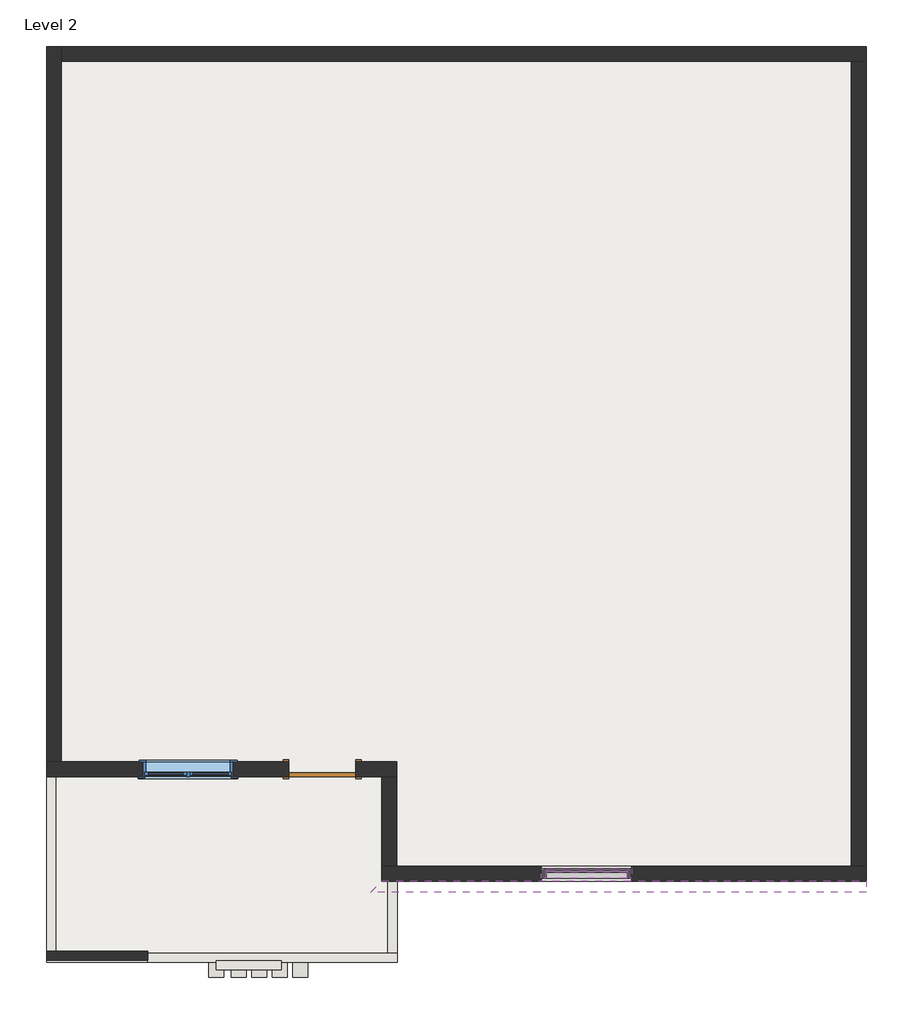
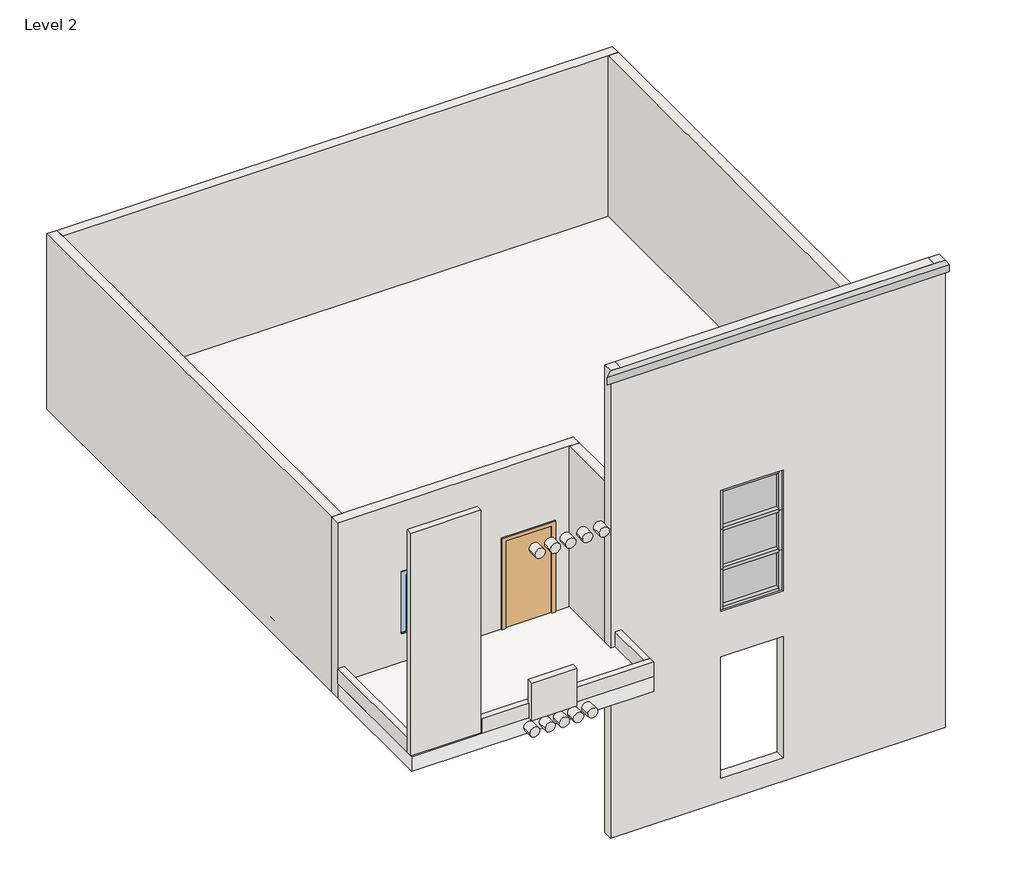
# One storey: 12 walls, 10 members, 3 plates, 1 door, 1 proxy, 1 roof, 1 window.
"""IFC4 building model written with IfcOpenShell, lengths in millimetres."""

from ifc_helpers import new_model, si_unit, frame, origin, place, context, project, spatial, polyline, outline, extrude, faceted_brep, transform, mapped, element, save
from components import door_54dd4da4, member_b365ec95, member_88401a07, member_a8c92c1b, system_panel_glazed_b873dfd1, system_panel_glazed_e970100d, walls_4_walls_4_cfa72774, window_0862ab64

model = new_model("IFC4")

# Units and contexts
model_context = context("Model", 3, world=origin())
ifc_project = project(units=[si_unit("LENGTHUNIT", "METRE", prefix="MILLI")], contexts=[model_context])

# Site, building, storey
site = spatial("IfcSite", under=ifc_project)
building = spatial("IfcBuilding", under=site)
storey = spatial("IfcBuildingStorey", under=building, Name="Level 2", Elevation=3657.6)

# Proxy
placement = place(None, origin())
element("IfcBuildingElementProxy", 1, Name="Cornice", ObjectType="Cornice", at=placement, inside=storey, context=model_context, shape_type="SweptSolid", body=[
    extrude(outline(polyline([(-6596.5183714, -375.7099629), (-6444.1183714, -223.3099629), (159.8816286, -223.3099629), (159.8816286, -375.7099629), (-6596.5183714, -375.7099629)])), frame((0.0, 0.0, 9601.2), z_axis=(0.0, 0.0, 1.0), x_axis=(1.0, 0.0, 0.0)), (0.0, 0.0, 1.0), 152.4),
])

# Door
door_shape = door_54dd4da4(model_context)
element("IfcDoor", 2, ObjectType="Single-Flush : 36\" x 84\"", at=placement, inside=storey, context=model_context, shape_type="MappedRepresentation", body=[
    mapped(door_shape, transform((-7256.9183714, 1300.6900371, 3657.6), x_axis=(-1.0, 0.0, 0.0), y_axis=(0.0, -1.0, 0.0), z_axis=(0.0, 0.0, 1.0))),
])

# Members
member_shape = member_b365ec95(model_context)
element("IfcMember", 3, ObjectType="Rectangular Mullion : 2.5\" x 5\" rectangular", at=placement, inside=storey, context=model_context, shape_type="MappedRepresentation", body=[
    mapped(member_shape, transform((-4267.1276154, -121.7099629, 5644.4580483), x_axis=(-1.0, 0.0, 0.0), y_axis=(0.0, -1.0, 0.0), z_axis=(0.0, 0.0, 1.0))),
])
element("IfcMember", 4, ObjectType="Rectangular Mullion : 2.5\" x 5\" rectangular", at=placement, inside=storey, context=model_context, shape_type="MappedRepresentation", body=[
    mapped(member_shape, transform((-4267.1276154, -121.7099629, 6485.4870724), x_axis=(-1.0, 0.0, 0.0), y_axis=(0.0, -1.0, 0.0), z_axis=(0.0, 0.0, 1.0))),
])
member_2_shape = member_88401a07(model_context)
element("IfcMember", 5, ObjectType="Rectangular Mullion : 2.5\" x 5\" rectangular", at=placement, inside=storey, context=model_context, shape_type="MappedRepresentation", body=[
    mapped(member_2_shape, transform((-3100.8433714, -121.7099629, 5644.4580483), x_axis=(0.0, 0.0, 1.0), y_axis=(0.0, -1.0, 0.0), z_axis=(1.0, 0.0, 0.0))),
])
element("IfcMember", 6, ObjectType="Rectangular Mullion : 2.5\" x 5\" rectangular", at=placement, inside=storey, context=model_context, shape_type="MappedRepresentation", body=[
    mapped(member_2_shape, transform((-3100.8433714, -121.7099629, 4803.4290241), x_axis=(0.0, 0.0, 1.0), y_axis=(0.0, -1.0, 0.0), z_axis=(1.0, 0.0, 0.0))),
])
member_3_shape = member_a8c92c1b(model_context)
element("IfcMember", 7, ObjectType="Rectangular Mullion : 2.5\" x 5\" rectangular", at=placement, inside=storey, context=model_context, shape_type="MappedRepresentation", body=[
    mapped(member_3_shape, transform((-3100.8433714, -121.7099629, 6485.4870724), x_axis=(0.0, 0.0, 1.0), y_axis=(0.0, -1.0, 0.0), z_axis=(1.0, 0.0, 0.0))),
])
element("IfcMember", 8, ObjectType="Rectangular Mullion : 2.5\" x 5\" rectangular", at=placement, inside=storey, context=model_context, shape_type="MappedRepresentation", body=[
    mapped(member_shape, transform((-3037.3433714, -121.7099629, 4803.4290241), x_axis=(1.0, 0.0, 0.0), y_axis=(0.0, -1.0, 0.0), z_axis=(0.0, 0.0, -1.0))),
])
element("IfcMember", 9, ObjectType="Rectangular Mullion : 2.5\" x 5\" rectangular", at=placement, inside=storey, context=model_context, shape_type="MappedRepresentation", body=[
    mapped(member_shape, transform((-3037.3433714, -121.7099629, 5644.4580483), x_axis=(1.0, 0.0, 0.0), y_axis=(0.0, -1.0, 0.0), z_axis=(0.0, 0.0, -1.0))),
])
element("IfcMember", 10, ObjectType="Rectangular Mullion : 2.5\" x 5\" rectangular", at=placement, inside=storey, context=model_context, shape_type="MappedRepresentation", body=[
    mapped(member_3_shape, transform((-4203.6276154, -121.7099629, 3962.4), x_axis=(0.0, 0.0, -1.0), y_axis=(0.0, -1.0, 0.0), z_axis=(-1.0, 0.0, 0.0))),
])
element("IfcMember", 11, ObjectType="Rectangular Mullion : 2.5\" x 5\" rectangular", at=placement, inside=storey, context=model_context, shape_type="MappedRepresentation", body=[
    mapped(member_shape, transform((-4267.1276154, -121.7099629, 4803.4290241), x_axis=(-1.0, 0.0, 0.0), y_axis=(0.0, -1.0, 0.0), z_axis=(0.0, 0.0, 1.0))),
])
element("IfcMember", 12, ObjectType="Rectangular Mullion : 2.5\" x 5\" rectangular", at=placement, inside=storey, context=model_context, shape_type="MappedRepresentation", body=[
    mapped(member_shape, transform((-3037.3433714, -121.7099629, 3962.4), x_axis=(1.0, 0.0, 0.0), y_axis=(0.0, -1.0, 0.0), z_axis=(0.0, 0.0, -1.0))),
])

# Plates
system_panel_glazed_shape = system_panel_glazed_b873dfd1(model_context)
element("IfcPlate", 13, ObjectType="System Panel : Glazed", at=placement, inside=storey, context=model_context, shape_type="MappedRepresentation", body=[
    mapped(system_panel_glazed_shape, transform((-3652.2354934, -121.7099629, 4025.9), x_axis=(1.0, 0.0, 0.0), y_axis=(0.0, 1.0, 0.0), z_axis=(0.0, 0.0, 1.0))),
])
element("IfcPlate", 14, ObjectType="System Panel : Glazed", at=placement, inside=storey, context=model_context, shape_type="MappedRepresentation", body=[
    mapped(system_panel_glazed_shape, transform((-3652.2354934, -121.7099629, 5676.2080483), x_axis=(1.0, 0.0, 0.0), y_axis=(0.0, 1.0, 0.0), z_axis=(0.0, 0.0, 1.0))),
])
system_panel_glazed_2_shape = system_panel_glazed_e970100d(model_context)
element("IfcPlate", 15, ObjectType="System Panel : Glazed", at=placement, inside=storey, context=model_context, shape_type="MappedRepresentation", body=[
    mapped(system_panel_glazed_2_shape, transform((-3652.2354934, -121.7099629, 4835.1790241), x_axis=(1.0, 0.0, 0.0), y_axis=(0.0, 1.0, 0.0), z_axis=(0.0, 0.0, 1.0))),
])

# Roof
element("IfcRoof", 16, ObjectType="Generic - 12\"", at=placement, inside=storey, context=model_context, shape_type="SweptSolid", body=[
    extrude(outline(polyline([(-11016.1183714, 11155.8900371), (159.8816286, 11155.8900371), (159.8816286, -20.1099629), (-6234.5683714, -20.1099629), (-6234.5683714, -1332.6895946), (-11016.1183714, -1332.6895946), (-11016.1183714, 11155.8900371)])), frame((0.0, 0.0, 3657.6), z_axis=(0.0, 0.0, 1.0), x_axis=(1.0, 0.0, 0.0)), (0.0, 0.0, 1.0), 304.8),
])

# Walls
element("IfcWall", 17, ObjectType="Generic - 5\"", at=placement, inside=storey, context=model_context, shape_type="Brep", body=[
    faceted_brep([(-11016.1183714, -1306.3008757, 8615.143067), (-11016.1183714, -1306.3008757, 3962.4), (-9633.3839949, -1306.3008757, 3962.4), (-9633.3839949, -1306.3008757, 8615.143067), (-11016.1183714, -1179.3008757, 3962.4), (-11016.1183714, -1179.3008757, 4267.2), (-11016.1183714, -1179.3008757, 7620.0), (-11016.1183714, -1179.3008757, 7924.8), (-11016.1183714, -1179.3008757, 8615.143067), (-9633.3839949, -1179.3008757, 8615.143067), (-9633.3839949, -1179.3008757, 3962.4), (-10889.1183714, -1179.3008757, 3962.4), (-9633.3839949, -1205.6895946, 3962.4)], [[[0, 1, 2, 3]], [[4, 5, 6, 7, 8, 9, 10, 11]], [[2, 1, 4, 11, 10, 12]], [[0, 3, 9, 8]], [[2, 12, 10, 9, 3]], [[0, 8, 7, 6, 5, 4, 1]]]),
])
element("IfcWall", 18, ObjectType="Generic - 5\"", at=placement, inside=storey, context=model_context, shape_type="Brep", body=[
    faceted_brep([(-9633.3839949, -1332.6895946, 3962.4), (-6234.5683714, -1332.6895946, 3962.4), (-6234.5683714, -1332.6895946, 4267.2), (-9633.3839949, -1332.6895946, 4267.2), (-9633.3839949, -1205.6895946, 3962.4), (-9633.3839949, -1205.6895946, 4267.2), (-6361.5683714, -1205.6895946, 4267.2), (-6234.5683714, -1205.6895946, 4267.2), (-6234.5683714, -1205.6895946, 3962.4), (-6361.5683714, -1205.6895946, 3962.4), (-9633.3839949, -1306.3008757, 3962.4)], [[[0, 1, 2, 3]], [[4, 5, 6, 7, 8, 9]], [[1, 0, 10, 4, 9, 8]], [[3, 2, 7, 6, 5]], [[0, 3, 5, 4, 10]], [[2, 1, 8, 7]]]),
])
element("IfcWall", 19, ObjectType="Generic - 5\"", at=placement, inside=storey, context=model_context, shape_type="SweptSolid", body=[
    extrude(outline(polyline([(-6234.5683714, -223.3099629), (-6234.5683714, -1205.6895946), (-6361.5683714, -1205.6895946), (-6361.5683714, -223.3099629), (-6234.5683714, -223.3099629)])), frame((0.0, 0.0, 3962.4), z_axis=(0.0, 0.0, 1.0), x_axis=(1.0, 0.0, 0.0)), (0.0, 0.0, 1.0), 304.8),
])
element("IfcWall", 20, ObjectType="Generic - 5\"", at=placement, inside=storey, context=model_context, shape_type="SweptSolid", body=[
    extrude(outline(polyline([(-11016.1183714, -1179.3008757), (-11016.1183714, 1199.0900371), (-10889.1183714, 1199.0900371), (-10889.1183714, -1179.3008757), (-11016.1183714, -1179.3008757)])), frame((0.0, 0.0, 3962.4), z_axis=(0.0, 0.0, 1.0), x_axis=(1.0, 0.0, 0.0)), (0.0, 0.0, 1.0), 304.8),
])
element("IfcWall", 21, ObjectType="Generic - 5\"", at=placement, inside=storey, context=model_context, shape_type="SweptSolid", body=[
    extrude(outline(polyline([(-7812.5433714, -1434.2895946), (-8701.5433714, -1434.2895946), (-8701.5433714, -1307.2895946), (-7812.5433714, -1307.2895946), (-7812.5433714, -1434.2895946)])), frame((0.0, 0.0, 3962.4), z_axis=(0.0, 0.0, 1.0), x_axis=(1.0, 0.0, 0.0)), (0.0, 0.0, 1.0), 788.2116103),
])
element("IfcWall", 22, ObjectType="Generic - 8\"", at=placement, inside=storey, context=model_context, shape_type="Brep", body=[
    faceted_brep([(-6444.1183714, -223.3099629, -11.5518253), (159.8816286, -223.3099629, -11.5518253), (159.8816286, -223.3099629, 9601.2), (159.8816286, -223.3099629, 9753.6), (-49.6683714, -223.3099629, 9753.6), (-6240.9183714, -223.3099629, 9753.6), (-6444.1183714, -223.3099629, 9753.6), (-6444.1183714, -223.3099629, 9601.2), (-3037.3433714, -223.3099629, 6485.4870724), (-3037.3433714, -223.3099629, 3962.4), (-4267.1276154, -223.3099629, 3962.4), (-4267.1276154, -223.3099629, 6485.4870724), (-3037.3433714, -223.3099629, 3011.0508937), (-3037.3433714, -223.3099629, 473.4885433), (-4267.1276154, -223.3099629, 473.4885433), (-4267.1276154, -223.3099629, 3011.0508937), (159.8816286, -20.1099629, -11.5518253), (-6444.1183714, -20.1099629, -11.5518253), (-6444.1183714, -20.1099629, 0.0), (-6444.1183714, -20.1099629, 3657.6), (-6444.1183714, -20.1099629, 7315.2), (-6444.1183714, -20.1099629, 9601.2), (-6444.1183714, -20.1099629, 9753.6), (-6240.9183714, -20.1099629, 9753.6), (-49.6683714, -20.1099629, 9753.6), (-43.3183714, -20.1099629, 9753.6), (159.8816286, -20.1099629, 9753.6), (159.8816286, -20.1099629, 7315.2), (159.8816286, -20.1099629, 3657.6), (159.8816286, -20.1099629, 0.0), (-3037.3433714, -20.1099629, 3962.4), (-3037.3433714, -20.1099629, 6485.4870724), (-4267.1276154, -20.1099629, 6485.4870724), (-4267.1276154, -20.1099629, 3962.4), (-3037.3433714, -20.1099629, 473.4885433), (-3037.3433714, -20.1099629, 3011.0508937), (-4267.1276154, -20.1099629, 3011.0508937), (-4267.1276154, -20.1099629, 473.4885433)], [[[0, 1, 2, 3, 4, 5, 6, 7], [8, 9, 10, 11], [12, 13, 14, 15]], [[16, 17, 18, 19, 20, 21, 22, 23, 24, 25, 26, 27, 28, 29], [30, 31, 32, 33], [34, 35, 36, 37]], [[16, 29, 28, 27, 26, 3, 2, 1]], [[17, 0, 7, 6, 22, 21, 20, 19, 18]], [[1, 0, 17, 16]], [[4, 3, 26, 25, 24]], [[24, 23, 5, 4]], [[23, 22, 6, 5]], [[9, 8, 31, 30]], [[10, 9, 30, 33]], [[11, 10, 33, 32]], [[8, 11, 32, 31]], [[13, 12, 35, 34]], [[14, 13, 34, 37]], [[15, 14, 37, 36]], [[12, 15, 36, 35]]]),
])
element("IfcWall", 23, ObjectType="Generic - 8\"", at=placement, inside=storey, context=model_context, shape_type="Brep", body=[
    faceted_brep([(-11016.1183714, 1199.0900371, 3657.6), (-7714.1183714, 1199.0900371, 3657.6), (-7714.1183714, 1199.0900371, 5791.2), (-6799.7183714, 1199.0900371, 5791.2), (-6799.7183714, 1199.0900371, 3657.6), (-6444.1183714, 1199.0900371, 3657.6), (-6240.9183714, 1199.0900371, 3657.6), (-6240.9183714, 1199.0900371, 7315.2), (-6444.1183714, 1199.0900371, 7315.2), (-11016.1183714, 1199.0900371, 7315.2), (-11016.1183714, 1199.0900371, 4267.2), (-11016.1183714, 1199.0900371, 3962.4), (-9695.3183714, 1199.0900371, 5791.2), (-8476.1183714, 1199.0900371, 5791.2), (-8476.1183714, 1199.0900371, 4572.0), (-9695.3183714, 1199.0900371, 4572.0), (-7714.1183714, 1402.2900371, 5791.2), (-7714.1183714, 1402.2900371, 3657.6), (-10812.9183714, 1402.2900371, 3657.6), (-11016.1183714, 1402.2900371, 3657.6), (-11016.1183714, 1402.2900371, 7315.2), (-10812.9183714, 1402.2900371, 7315.2), (-6240.9183714, 1402.2900371, 7315.2), (-6240.9183714, 1402.2900371, 3657.6), (-6799.7183714, 1402.2900371, 3657.6), (-6799.7183714, 1402.2900371, 5791.2), (-9695.3183714, 1402.2900371, 5791.2), (-9695.3183714, 1402.2900371, 4572.0), (-8476.1183714, 1402.2900371, 4572.0), (-8476.1183714, 1402.2900371, 5791.2)], [[[0, 1, 2, 3, 4, 5, 6, 7, 8, 9, 10, 11], [12, 13, 14, 15]], [[16, 17, 18, 19, 20, 21, 22, 23, 24, 25], [26, 27, 28, 29]], [[24, 23, 6, 5, 4]], [[19, 18, 17, 1, 0]], [[9, 8, 7, 22, 21, 20]], [[7, 6, 23, 22]], [[9, 20, 19, 0, 11, 10]], [[2, 1, 17, 16]], [[3, 2, 16, 25]], [[4, 3, 25, 24]], [[27, 26, 12, 15]], [[28, 27, 15, 14]], [[29, 28, 14, 13]], [[26, 29, 13, 12]]]),
])
element("IfcWall", 24, ObjectType="Generic - 8\"", at=placement, inside=storey, context=model_context, shape_type="Brep", body=[
    faceted_brep([(-10812.9183714, 1402.2900371, 7315.2), (-10812.9183714, 1402.2900371, 3657.6), (-10812.9183714, 10952.6900371, 3657.6), (-10812.9183714, 11155.8900371, 3657.6), (-10812.9183714, 11155.8900371, 7315.2), (-10812.9183714, 10952.6900371, 7315.2), (-11016.1183714, 1402.2900371, 3657.6), (-11016.1183714, 1402.2900371, 7315.2), (-11016.1183714, 11155.8900371, 7315.2), (-11016.1183714, 11155.8900371, 3657.6)], [[[0, 1, 2, 3, 4, 5]], [[6, 7, 8, 9]], [[3, 2, 1, 6, 9]], [[0, 5, 4, 8, 7]], [[4, 3, 9, 8]], [[0, 7, 6, 1]]]),
])
element("IfcWall", 25, ObjectType="Generic - 8\"", at=placement, inside=storey, context=model_context, shape_type="Brep", body=[
    faceted_brep([(-10812.9183714, 10952.6900371, 3657.6), (-43.3183714, 10952.6900371, 3657.6), (159.8816286, 10952.6900371, 3657.6), (159.8816286, 10952.6900371, 7315.2), (-43.3183714, 10952.6900371, 7315.2), (-10812.9183714, 10952.6900371, 7315.2), (-10812.9183714, 11155.8900371, 3657.6), (-10812.9183714, 11155.8900371, 7315.2), (159.8816286, 11155.8900371, 7315.2), (159.8816286, 11155.8900371, 3657.6)], [[[0, 1, 2, 3, 4, 5]], [[6, 7, 8, 9]], [[2, 1, 0, 6, 9]], [[5, 4, 3, 8, 7]], [[0, 5, 7, 6]], [[3, 2, 9, 8]]]),
])
element("IfcWall", 26, ObjectType="Generic - 8\"", at=placement, inside=storey, context=model_context, shape_type="Brep", body=[
    faceted_brep([(-43.3183714, 10952.6900371, 3657.6), (-43.3183714, -20.1099629, 3657.6), (-43.3183714, -20.1099629, 7315.2), (-43.3183714, 5567.8900371, 7315.2), (-43.3183714, 10952.6900371, 7315.2), (159.8816286, 10952.6900371, 3657.6), (159.8816286, 10952.6900371, 7315.2), (159.8816286, 5567.8900371, 7315.2), (159.8816286, -20.1099629, 7315.2), (159.8816286, -20.1099629, 3657.6)], [[[0, 1, 2, 3, 4]], [[5, 6, 7, 8, 9]], [[1, 0, 5, 9]], [[4, 3, 2, 8, 7, 6]], [[2, 1, 9, 8]], [[0, 4, 6, 5]]]),
])
element("IfcWall", 27, ObjectType="Generic - 8\"", at=placement, inside=storey, context=model_context, shape_type="SweptSolid", body=[
    extrude(outline(polyline([(-6444.1183714, -20.1099629), (-6444.1183714, 1199.0900371), (-6240.9183714, 1199.0900371), (-6240.9183714, -20.1099629), (-6444.1183714, -20.1099629)])), frame((0.0, 0.0, 3657.6), z_axis=(0.0, 0.0, 1.0), x_axis=(1.0, 0.0, 0.0)), (0.0, 0.0, 1.0), 3657.6),
])
walls_4_walls_4_shape = walls_4_walls_4_cfa72774(model_context)
element("IfcWall", 28, ObjectType="Walls 4 : Walls 4", at=placement, inside=storey, context=model_context, shape_type="MappedRepresentation", body=[
    mapped(walls_4_walls_4_shape, transform((0.0, 0.0, 0.0), x_axis=(1.0, 0.0, 0.0), y_axis=(0.0, 1.0, 0.0), z_axis=(0.0, 0.0, 1.0))),
])

# Window
window_shape = window_0862ab64(model_context)
element("IfcWindow", 29, ObjectType="Casement Dbl with Trim.0001 : 48\" x 48\"", at=placement, inside=storey, context=model_context, shape_type="MappedRepresentation", body=[
    mapped(window_shape, transform((-9085.7183714, 1319.7400371, 3657.6), x_axis=(-1.0, 0.0, 0.0), y_axis=(0.0, -1.0, 0.0), z_axis=(0.0, 0.0, 1.0))),
])

save(model, "model.ifc")

# Revit data of these elements
# Type "Single-Flush : 36\" x 84\""
#   Type Mark = "1"
#   Construction Type Id = "MDOOR"
#   Assembly Code = "C1020"
#   Analytic Construction = "Metal"
#   Thickness = 0' - 2"
#   Heat Transfer Coefficient (U) = 0.651978 BTU/(h·ft²·°F)
#   Height = 7' - 0"
#   Trim Projection Ext = 0' - 1"
#   Trim Projection Int = 0' - 1"
#   Trim Width = 0' - 3"
#   Width = 3' - 0"
#   Define Thermal Properties by = 1
#   Door Material = Door - Panel
#   Frame Material = Door - Frame
#   Visual Light Transmittance = 0
#   Solar Heat Gain Coefficient = 0
#   Function = (empty or 0)
#   Wall Closure = (empty or 0)
# Type "Rectangular Mullion : 2.5\" x 5\" rectangular"
#   built-in parameter 1007304 = 0.416667 (stored number, unit not read)
#   built-in parameter 1007301 = 0.104167 (stored number, unit not read)
#   built-in parameter 1007300 = 0.104167 (stored number, unit not read)
# Type "System Panel : Glazed"
#   Construction Type Id = "GSP4R"
#   Analytic Construction = "1/8 in Pilkington single glazing"
#   Visual Light Transmittance = 0.9
#   Solar Heat Gain Coefficient = 0.86
#   Heat Transfer Coefficient (U) = 1.18115 BTU/(h·ft²·°F)
# Type "Generic - 12\""
#   Assembly Code = "B1020"
#   Layers, outside or top first: 1' - 0" no material (function 1)
# Type "Generic - 5\""
#   Assembly Code = "B2010"
#   Layers, outside or top first: 0' - 5" no material (function 1)
# Type "Generic - 8\""
#   Assembly Code = "B2010"
#   Layers, outside or top first: 0' - 8" no material (function 1)
# Type "Casement Dbl with Trim.0001 : 48\" x 48\""
#   Type Mark = "10"
#   Construction Type Id = "GSP4R"
#   Assembly Code = "B2020100"
#   Analytic Construction = "1/8 in Pilkington single glazing"
#   Visual Light Transmittance = 0.9
#   Solar Heat Gain Coefficient = 0.78
#   Heat Transfer Coefficient (U) = 0.6496 BTU/(h·ft²·°F)
#   Height = 4' - 0"
#   Default Sill Height = 3' - 0"
#   Trim Projection - Ext. = 0' - 0 1/2"
#   Trim Projection - Int. = 0' - 0 3/4"
#   Trim Width - Exterior = 0' - 3 1/2"
#   Trim Width - Interior = 0' - 3 1/2"
#   Width = 4' - 0"
#   Window Inset = 0' - 0 3/4"
#   Define Thermal Properties by = 1
#   Glass Pane Material = Glass
#   Sash Material = Sash
#   Trim Exterior Material = Trim
#   Trim Interior Material = Trim
#   Wall Closure = (empty or 0)
# Element 1 (IfcBuildingElementProxy, "Cornice")
#   Phase Created = New Construction
#   Materials on its faces: "Default Wall"
# Element 2 (IfcDoor, "Single-Flush : 36\" x 84\"")
#   Phase Created = New Construction
#   Materials on its faces: "Door - Frame", "Door - Panel"
# Elements 3, 4, 5, 6, 7, 8, 9, 10, 11, 12 (IfcMember, "Rectangular Mullion : 2.5\" x 5\" rectangular")
#   Phase Created = New Construction
#   Materials on its faces: "Aluminum"
# Elements 13, 14, 15 (IfcPlate, "System Panel : Glazed")
#   Phase Created = New Construction
#   Materials on its faces: "Glass"
# Element 16 (IfcRoof, "Generic - 12\"")
#   built-in parameter 1001705 = 13 (stored number, unit not read)
#   built-in parameter 1001710 = 33615
#   Phase Created = New Construction
#   Materials on its faces: "Default Roof"
# Element 17 (IfcWall, "Generic - 5\"")
#   built-in parameter 1001111 = 1' - 0"
#   Top Offset = 4' - 3.17886"
#   Base Offset = 1' - 0"
#   wall height = 15' - 3.17886"
#   Phase Created = New Construction
#   Base Constraint = Level 2
#   Top Constraint = Level 3
#   Materials on its faces: "Default Wall"
# Elements 18, 19, 20 (IfcWall, "Generic - 5\"")
#   built-in parameter 1001111 = 1' - 0"
#   Top Offset = -10' - 0"
#   Base Offset = 1' - 0"
#   wall height = 1' - 0"
#   Phase Created = New Construction
#   Base Constraint = Level 2
#   Top Constraint = Level 3
#   Materials on its faces: "Default Wall"
# Element 21 (IfcWall, "Generic - 5\"")
#   built-in parameter 1001111 = 1' - 0"
#   Top Offset = -8' - 4.96805"
#   Base Offset = 1' - 0"
#   wall height = 2' - 7.03195"
#   Phase Created = New Construction
#   Base Constraint = Level 2
#   Top Constraint = Level 3
#   Materials on its faces: "Default Wall"
# Element 22 (IfcWall, "Generic - 8\"")
#   built-in parameter 1001111 = -12' - 0.4548"
#   Top Offset = 0' - 0"
#   Base Offset = -12' - 0.4548"
#   Unconnected Height = 32' - 0.4548"
#   wall height = 32' - 0.4548"
#   Phase Created = New Construction
#   Base Constraint = Level 2
#   Materials on its faces: "Default Wall"
# Elements 23, 24, 25, 26, 27 (IfcWall, "Generic - 8\"")
#   Top Offset = 0' - 0"
#   Base Offset = 0' - 0"
#   Unconnected Height = 12' - 0"
#   wall height = 12' - 0"
#   Phase Created = New Construction
#   Base Constraint = Level 2
#   Materials on its faces: "Default Wall"
# Element 28 (IfcWall, "Walls 4 : Walls 4")
#   Phase Created = New Construction
#   Materials on its faces: "Default Wall"
# Element 29 (IfcWindow, "Casement Dbl with Trim.0001 : 48\" x 48\"")
#   Mark = "1"
#   Phase Created = New Construction
#   Materials on its faces: "Sash", "Trim", "Glass"
# Materials
#   "Door - Panel": class "Wood", colour RGB 210 159 95, transparency 0
#   "Door - Frame": colour RGB 118 70 51, transparency 0
#   "Glass": class "Glass", colour RGB 0 128 192, transparency 0.75, Description = "Soda Lime Glass", Cost = 0
#   "Sash": class "Wood", colour RGB 224 178 126, transparency 0
#   "Trim": class "Wood", colour RGB 224 178 126, transparency 0
#   "Default Wall": colour RGB 128 128 128, transparency 0
#   "Aluminum": class "Metal", colour RGB 247 247 247, transparency 0, Description = "Aluminum 6061", Cost = 0
#   "Default Roof": colour RGB 88 101 114, transparency 0
